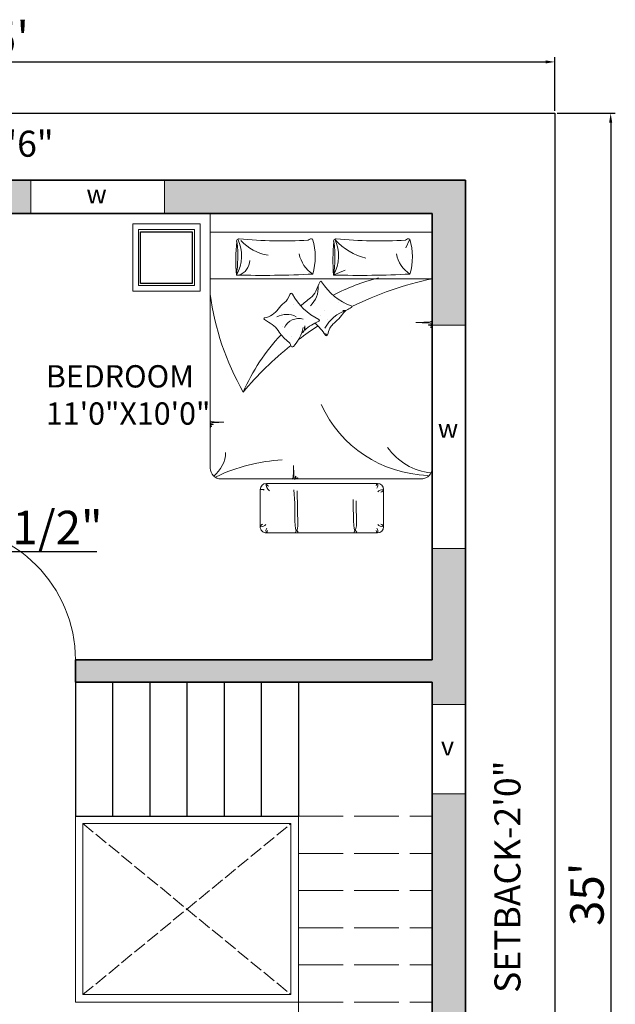
# Model space of a CAD drawing. Units: inches. Extents: x 3488 to 4319, y 780 to 1756.
# Tile 5 of 8: x 3679 to 3839, y 1491 to 1756. Entities that reach past the tile are written whole.
import ezdxf

# ---------------------------------------------------------------- set-up
doc = ezdxf.new("R2010")
doc.units = ezdxf.units.IN
doc.linetypes.add('ACAD_ISO02W100', pattern=[15, 12, -3])
for name, color, linetype, lineweight in [('A-ANNO-IDEN', 7, 'Continuous', 13), ('A-ANNO-TEXT', 7, 'Continuous', 18), ('A-AREA-IDEN', 7, 'Continuous', 18), ('A-DOOR', 4, 'Continuous', 18), ('A-FLOR-OPEN', 3, 'Continuous', 20), ('A-FLOR-OPEN-HIDN', 3, 'ACAD_ISO02W100', 13), ('A-FLOR-STRS', 7, 'Continuous', 25), ('A-FLOR-STRS-OVHD', 8, 'ACAD_ISO02W100', 18), ('A-WALL', 7, 'Continuous', 35), ('A-WALL-PATT', 252, 'Continuous', 13), ('C-PROP', 7, 'Continuous', 25), ('DIM', 9, 'Continuous', 18), ('FUR', 42, 'Continuous', 18), ('window', 130, 'Continuous', 18)]:
    doc.layers.add(name, color=color, linetype=linetype, lineweight=lineweight)
doc.layers.add('HA-FUR', color=8, linetype='Continuous')
doc.layers.add('wood', color=26, linetype='Continuous')
doc.styles.get("Standard").update_dxf_attribs({"font": 'arial.ttf'})
doc.dimstyles.new('ISO-25', dxfattribs={"dimtxt": 9, "dimasz": 2.5, "dimexe": 1.25, "dimexo": 0.625, "dimtad": 1, "dimdec": 1, "dimlunit": 3, "dimtxsty": 'Standard', "dimcen": 2.5, "dimclrd": 1, "dimclre": 1, "dimclrt": 1, "dimadec": 0, "dimazin": 0, "dimtfac": 1, "dimtdec": 1, "dimtmove": 0, "dimatfit": 3, "dimfxl": 1, "dimarcsym": 0})

# ---------------------------------------------------------------- blocks, each defined once
blk = doc.blocks.new('*U3')
for p, q in [((0, 0), (0, -6)), ((36, 0), (36, -6))]:
    blk.add_line(p, q)
blk.add_lwpolyline([(0, 0), (0, 36), (1.75, 36), (1.75, 0)], close=True)
blk.add_arc((0, 0), 36, 0, 90)
blk = doc.blocks.new('*D5')
at = {"layer": 'Defpoints', "color": 0, "transparency": 16777216}
for p in [(3822.99, 1744.35), (3522.99, 1730.55), (3822.99, 1730.55)]:
    blk.add_point(p, dxfattribs=at)
at = {"layer": 'DIM', "color": 0, "lineweight": -2, "transparency": 16777216}
for p, q in [((3522.99, 1731.18), (3522.99, 1745.6)), ((3822.99, 1731.18), (3822.99, 1745.6)), ((3525.49, 1744.35), (3820.49, 1744.35))]:
    blk.add_line(p, q, dxfattribs=at)
at = {"layer": 'DIM', "color": 0, "transparency": 16777216}
for points in [[(3525.49, 1744.77), (3525.49, 1743.94), (3522.99, 1744.35)], [(3820.49, 1744.77), (3820.49, 1743.94), (3822.99, 1744.35)]]:
    blk.add_solid(points, dxfattribs=at)
at = {"layer": 'DIM', "color": 0, "transparency": 16777216, "insert": (3672.99, 1749.57), "char_height": 9, "attachment_point": 5}
blk.add_mtext("25'", dxfattribs=at)
blk = doc.blocks.new('*D6')
at = {"layer": 'Defpoints', "color": 0, "transparency": 16777216}
for p in [(3822.99, 1730.55), (3822.99, 1310.55), (3838.01, 1310.55)]:
    blk.add_point(p, dxfattribs=at)
at = {"layer": 'DIM', "color": 0, "lineweight": -2, "transparency": 16777216}
for p, q in [((3823.61, 1730.55), (3839.26, 1730.55)), ((3838.01, 1728.05), (3838.01, 1313.05)), ((3823.61, 1310.55), (3839.26, 1310.55))]:
    blk.add_line(p, q, dxfattribs=at)
at = {"layer": 'DIM', "color": 0, "transparency": 16777216}
for points in [[(3837.59, 1728.05), (3838.43, 1728.05), (3838.01, 1730.55)], [(3837.59, 1313.05), (3838.43, 1313.05), (3838.01, 1310.55)]]:
    blk.add_solid(points, dxfattribs=at)
at = {"layer": 'DIM', "color": 0, "transparency": 16777216, "insert": (3832.79, 1520.55), "char_height": 9, "attachment_point": 5, "rotation": 90}
blk.add_mtext("35'", dxfattribs=at)
blk = doc.blocks.new('*X27')
at = {"color": 0}
for p, q in [((3147.8, 8143.4), (3147.8, 8143.4)), ((3155.9, 8182.9), (3155.9, 8182.9)), ((3209.5, 8023.9), (3209.5, 8023.9)), ((3251.6, 7997), (3251.6, 7997)), ((3283, 8049.6), (3283, 8049.6)), ((3154.1, 7950.7), (3154.1, 7950.7))]:
    blk.add_line(p, q, dxfattribs=at)
blk = doc.blocks.new('*X26')
at = {"color": 0}
for p, q in [((3155.9, 8182.9), (3155.9, 8182.9)), ((3139.8, 7939.7), (3139.8, 7939.7))]:
    blk.add_line(p, q, dxfattribs=at)
blk = doc.blocks.new('*X25')
at = {"color": 0}
for p, q in [((3155.9, 8182.9), (3155.9, 8182.9)), ((3139.8, 7939.7), (3139.8, 7939.7))]:
    blk.add_line(p, q, dxfattribs=at)
blk = doc.blocks.new('*X24')
at = {"color": 0}
for p, q in [((3163, 7776.2), (3163, 7776.2)), ((3422.2, 7761.3), (3422.2, 7761.3)), ((3236.2, 7675.7), (3236.2, 7675.7)), ((3244.3, 7698.6), (3244.3, 7698.6)), ((3340.3, 7689.4), (3340.3, 7689.4))]:
    blk.add_line(p, q, dxfattribs=at)
blk = doc.blocks.new('BED1')
for p, q in [((0, -1000), (0, 800)), ((150, 800), (0, 800)), ((150, 800), (150, -1000)), ((2058.7, 800), (150, 800)), ((528, 800), (528, -1000)), ((211.8, 614.9), (277.5, 585.4)), ((2537.2, 404.9), (2237.2, 404.9)), ((2187.2, 354.9), (2187.2, -545.1)), ((2587.2, -545.1), (2587.2, 354.9)), ((2566.3, 178.5), (2565.2, 177.4)), ((2582, 188.1), (2565.4, 174.8)), ((2565.4, 174.8), (2585.7, 165.4)), ((2566.3, -296.8), (2565.2, -297.9)), ((2582, -287.1), (2565.4, -300.5)), ((2565.4, -300.5), (2585.7, -309.9)), ((2237.2, -595.1), (2537.2, -595.1)), ((150, -1000), (0, -1000)), ((150, -1000), (2063.5, -1000))]:
    blk.add_line(p, q)
for points in [[(934, 797.9), (930.9, 797.7), (928.3, 797.4), (926.3, 796.9), (924.9, 796.3), (923.8, 795.6), (923.1, 794.8), (922.7, 793.8), (922.5, 792.7), (922.4, 791.5), (922.5, 790.3), (922.6, 789.2), (922.6, 788.3), (922.6, 787.6), (922.4, 787.3), (922, 787.4), (921.4, 787.9), (920.6, 788.9), (919.5, 790.2), (918.4, 791.6), (917.1, 793.1), (915.9, 794.6), (914.6, 796), (913.3, 797.1), (912.2, 797.9), (911.1, 798.3), (910.1, 798.4), (909.2, 798), (908.3, 797.1), (907.5, 795.8), (906.8, 793.9), (906, 791.4), (905.4, 788.5), (904.8, 785.2), (904.2, 781.7), (903.7, 778.4), (903.2, 775.4), (902.8, 772.9), (902.5, 771.3), (902.3, 770.6), (902.1, 771.2), (902, 772.8), (901.8, 775.2), (901.7, 778.1), (901.5, 781.5), (901.2, 785), (900.8, 788.4), (900.2, 791.5), (899.5, 794.1), (898.6, 796.2), (897.6, 797.9), (896.5, 799.2), (895.3, 800), (894.1, 800.5), (893, 800.7), (891.9, 800.5), (890.9, 800.1), (890, 799), (889.1, 797.1), (888.3, 794), (887.6, 789.3), (886.9, 782.9), (886.2, 774.2), (885.5, 763.1), (884.8, 749.5), (884.2, 734.2), (883.6, 718.3), (883, 702.8), (882.5, 688.8), (882, 677.5), (881.7, 669.8), (881.5, 666.9), (881.3, 669.4), (881.3, 676.7), (881.3, 687.8), (881.2, 701.5), (881.1, 716.8), (880.8, 732.6), (880.2, 748), (879.4, 761.8), (878.3, 773.2), (876.9, 782.2), (875.1, 789.2), (872.9, 794.4), (870.3, 798), (869, 799)], [(2150, -913.5), (2150, 723.2)], [(2327.6, 182.3), (2530, 185.9), (2550.8, 181.9), (2561.7, 179), (2566, 176.7), (2566.9, 174.4), (2566.3, 171.9), (2562, 169.2), (2550.3, 166.5), (2527.7, 163.9), (2490.6, 161.8), (2345.5, 160.2), (2317.8, 158.5)], [(494.7, 3.1), (458.9, 95.3)], [(2149.7, -259.9), (2150, -268.4), (2150.1, -274.1), (2150.1, -278.1), (2150, -281.4), (2149.8, -284), (2149.5, -286.1), (2149.1, -287.8), (2148.7, -289), (2148.1, -289.9), (2147.4, -290.5), (2146.6, -290.8), (2145.6, -291), (2144.6, -291), (2143.6, -291), (2142.7, -290.9), (2141.9, -290.9), (2141.4, -290.9), (2141.1, -291), (2141.2, -291.4), (2141.7, -291.9), (2142.5, -292.6), (2143.5, -293.4), (2144.7, -294.4), (2146, -295.4), (2147.2, -296.5), (2148.4, -297.6), (2149.3, -298.6), (2150, -299.6), (2150.3, -300.5), (2150.4, -301.3), (2150, -302.1), (2149.3, -302.8), (2148.2, -303.5), (2146.6, -304.1), (2144.6, -304.7), (2142.1, -305.2), (2139.3, -305.7), (2136.5, -306.2), (2133.7, -306.6), (2131.2, -307), (2129.2, -307.3), (2127.8, -307.6), (2127.3, -307.8), (2127.7, -308), (2129, -308.1), (2131, -308.2), (2133.5, -308.3), (2136.3, -308.5), (2139.2, -308.7), (2142, -309), (2144.6, -309.5), (2146.8, -310.1), (2148.6, -310.9), (2150, -311.7), (2151, -312.7), (2151.7, -313.6), (2152.1, -314.6), (2152.3, -315.6), (2152.2, -316.5), (2151.8, -317.3), (2150.9, -318.1), (2149.3, -318.8), (2146.7, -319.4), (2142.8, -320), (2137.4, -320.6), (2130.2, -321.2), (2121, -321.8), (2109.7, -322.3), (2096.9, -322.9), (2083.6, -323.4), (2070.7, -323.9), (2059.1, -324.3), (2049.6, -324.7), (2043.2, -325), (2040.8, -325.2), (2042.9, -325.3), (2049, -325.3), (2058.2, -325.3), (2069.6, -325.4), (2082.3, -325.5), (2095.6, -325.8), (2108.4, -326.2), (2119.9, -326.8), (2129.4, -327.8), (2136.9, -329), (2142.7, -330.5), (2147, -332.3), (2150, -334.4), (2150.9, -335.6)], [(2246.5, -294.4), (2530, -289.4), (2550.8, -293.4), (2561.7, -296.3), (2566, -298.6), (2566.9, -300.8), (2566.3, -303.4), (2562, -306.1), (2550.3, -308.8), (2527.7, -311.3), (2490.6, -313.5), (2345.5, -315), (2238.6, -321.8)], [(1733.7, -998.3), (1731.1, -998.1), (1729, -997.8), (1727.4, -997.4), (1726.1, -997), (1725.2, -996.4), (1724.7, -995.7), (1724.3, -994.8), (1724.1, -993.9), (1724.1, -992.9), (1724.1, -991.9), (1724.2, -991), (1724.2, -990.2), (1724.2, -989.7), (1724.1, -989.4), (1723.8, -989.5), (1723.2, -990), (1722.5, -990.8), (1721.7, -991.8), (1720.7, -993), (1719.7, -994.3), (1718.6, -995.5), (1717.5, -996.6), (1716.5, -997.6), (1715.5, -998.3), (1714.6, -998.6), (1713.8, -998.6), (1713, -998.3), (1712.3, -997.6), (1711.7, -996.5), (1711, -994.9), (1710.4, -992.9), (1709.9, -990.4), (1709.4, -987.6), (1708.9, -984.8), (1708.5, -982), (1708.1, -979.5), (1707.8, -977.4), (1707.5, -976.1), (1707.3, -975.5), (1707.1, -976), (1707, -977.3), (1706.9, -979.3), (1706.8, -981.8), (1706.7, -984.6), (1706.4, -987.5), (1706.1, -990.3), (1705.6, -992.9), (1705, -995.1), (1704.2, -996.9), (1703.4, -998.3), (1702.4, -999.3), (1701.5, -1000), (1700.5, -1000.4), (1699.6, -1000.6), (1698.7, -1000.4), (1697.8, -1000.1), (1697, -999.2), (1696.3, -997.6), (1695.7, -995), (1695.1, -991.1), (1694.5, -985.7), (1693.9, -978.5), (1693.3, -969.3), (1692.8, -957.9), (1692.2, -945.2), (1691.7, -931.9), (1691.2, -919), (1690.8, -907.4), (1690.4, -897.9), (1690.1, -891.5), (1689.9, -889.1), (1689.8, -891.2), (1689.8, -897.3), (1689.8, -906.5), (1689.7, -917.9), (1689.6, -930.6), (1689.4, -943.8), (1688.9, -956.6), (1688.3, -968.1), (1687.3, -977.6), (1686.1, -985.2), (1684.6, -991), (1682.8, -995.3), (1680.7, -998.3), (1679.6, -999.2)]]:
    blk.add_lwpolyline(points)
for points in [[(489.2, 619.6, 0.144019), (207.6, 617.9, 0.248643)], [(205.5, 619.6, 0.267769), (215.1, 582.4, -0.037739), (204.3, 21.8, 0.684696), (236.7, 5.5, -0.060702), (497.2, 0.1, -0.046649), (225.9, 3.1, -1.318436)], [(497.2, 0.1, 0.021276), (489.2, 619.6, -0.206383), (326.6, 509.4, 0.237198)], [(211.8, 12.8, 0.143972), (361.6, 262.9, 1.292232)], [(886.4, -150, -0.069098), (985, -66.5, 0.658965), (982.1, -48.7, -0.049789), (927.4, -29, -0.103757), (896.6, -5.4, 0.055725), (800.9, 83.3, -0.11866), (782.7, 104.9, 0.016811), (761.6, 143.9, 0.70791), (748.3, 144, -0.16964), (551.9, -96.6, 0.664036), (554, -110.7, 0.023706), (627, -144.7, -0.134834), (683.2, -188, 0.012748), (746.3, -267.4)], [(489.2, -168.2, 0.144019), (207.6, -169.9, 0.248643)], [(969.1, -259.1, 0.263265), (936.3, -236.9, -0.026108), (909.2, -233.2, 0.027613), (945.1, -234.2, -0.089259), (872.7, -120, 0.662242), (857.6, -119.3, -0.162037), (651.8, -332.7, 0.676499), (654, -354.5, -0.160513), (722.9, -401.5, 0.07473), (773.5, -450.3, -0.187721), (845.5, -559.9, 0.70791), (858.8, -561.4, -0.010003), (898.6, -497.3, -0.113819), (947.3, -450.2, 0.099539), (1032.5, -372.4, -0.173425), (1070.9, -346.4, 0.589988), (1076.2, -326.1, 0.137312), (923.9, -245.9, 0.137312)], [(205.5, -168.2, 0.267769), (215.1, -205.4, -0.037739), (204.3, -766, 0.684696), (236.7, -782.3, -0.060702), (497.2, -787.7, -0.046649), (225.9, -784.7, -1.318436)], [(497.2, -787.7, 0.021276), (489.2, -168.2, -0.206383), (326.6, -278.4, 0.237198)], [(1446, -733.4, -0.095039), (652.8, -1001.7)]]:
    blk.add_lwpolyline(points, format="xyb")
for centre, radius, start, end in [((3208.8, 1363.3), 2739.4, 191.86791, 206.32469), ((2062.7, 713.7), 86.5, 0, 93.53765), ((1138.6, 793.9), 983.2, 294.60777, 358.30329), ((1608.1, 842.5), 496.3, 305.19014, 354.02057), ((2237.2, 354.9), 50, 90, 180), ((2321.1, 409.7), 84.5, 185.61958, 217.13957), ((2227.5, 373.5), 32.8, 17.83305, 72.80048), ((2546.9, 373.5), 32.8, 107.19952, 162.16695), ((2453.3, 409.7), 84.5, 322.86043, 354.38042), ((2537.2, 354.9), 50, 0, 90), ((2098.7, 754.7), 1625, 193.90497, 207.81692), ((2201.9, 323.3), 34.8, 50.8413, 114.9586), ((2212.2, 381.5), 36.5, 226.80948, 258.3841), ((2572.5, 323.3), 34.8, 65.0414, 129.1587), ((2562.2, 381.5), 36.5, 281.6159, 313.19052), ((751.8, 88.7), 34.9, 336.83517, 27.72181), ((684.2, 86), 100.3, 353.675, 10.88198), ((1074.1, 198.8), 306.1, 197.86019, 241.51221), ((341.4, -277.7), 318.5, 60.71255, 115.00895), ((983.7, -79.5), 20.8, 73.79673, 130.45661), ((978.5, -68.6), 14.3, 39.7097, 85.9506), ((602.5, -324), 198.6, 43.20348, 95.05559), ((3208.8, 1363.3), 2739.4, 212.93136, 216.95099), ((980, -379), 163.4, 152.61037, 209.36102), ((981.1, -281.8), 131.1, 164.0372, 243.45361), ((3208.8, 1363.3), 2739.4, 218.63292, 229.94485), ((2098.7, 754.7), 1625, 226.58872, 246.3156), ((3402.5, -342.9), 1408.5, 182.99169, 205.68187), ((-34.4, -471.2), 376.5, 312.01178, 350.96348), ((2178, -513.5), 33, 286.18268, 338.13858), ((2237.2, -545.1), 50, 180, 270), ((2188.1, -476.2), 73, 269.45125, 322.80265), ((2453.3, -600), 84.5, 5.61958, 37.13957), ((2537.2, -545.1), 50, 270, 0), ((2572.5, -513.6), 34.8, 230.8413, 294.9586), ((2562.2, -571.8), 36.5, 46.80948, 78.3841), ((2271.1, -580.9), 35.8, 148.90546, 197.55407), ((2546.9, -563.8), 32.8, 197.83305, 252.80048), ((375.7, -807.4), 128.2, 17.40732, 88.51286), ((341.4, -1065.5), 318.5, 60.71255, 115.00895), ((1929.1, -1126), 250.5, 37.85533, 88.44053), ((2063.5, -913.5), 86.5, 270, 0)]:
    blk.add_arc(centre, radius, start, end)
for name in ['*X26', '*X25', '*X27', '*X24']:
    blk.add_blockref(name, (-2425.3, -8101.4))
blk = doc.blocks.new('A$C647F3D92')
at = {"layer": 'FUR'}
for points in [[(0.6, 0.6), (0, 0.6), (0, 0), (0.6, 0)], [(0.55, 0.55), (0.05, 0.55), (0.05, 0.05), (0.55, 0.05)]]:
    blk.add_lwpolyline(points, close=True, dxfattribs=at)
at = {"layer": 'HA-FUR'}
blk.add_lwpolyline([(0.53, 0.53), (0.07, 0.53), (0.07, 0.07), (0.53, 0.07)], close=True, dxfattribs=at)
blk = doc.blocks.new('A$C38A85F6B')
at = {"layer": 'wood', "xscale": -1, "rotation": 359.9999999999109}
blk.add_blockref('A$C647F3D92', (0.6, 0), dxfattribs=at)
blk = doc.blocks.new('STAIR-GROUND-LOWER-FLIGHT')
for p, q in [((0, 36), (0, 0)), ((10, 36), (10, 0)), ((20, 36), (20, 0)), ((30, 36), (30, 0)), ((40, 36), (40, 0)), ((50, 36), (50, 0)), ((60, 36), (60, 0)), ((0, 0), (60, 0))]:
    blk.add_line(p, q)
blk = doc.blocks.new('STAIR-GROUND-OVERHEAD-FLIGHT')
for p, q in [((0, 86), (0, 0)), ((0, 86), (36, 86)), ((0, 76), (36, 76)), ((0, 66), (36, 66)), ((0, 56), (36, 56)), ((0, 46), (36, 46)), ((0, 36), (36, 36)), ((0, 0), (36, 0))]:
    blk.add_line(p, q)
blk = doc.blocks.new('OPENING-STAIRWELL-FRAME')
for points in [[(60, 50), (0, 50), (0, 0), (60, 0)], [(58, 48), (2, 48), (2, 2), (58, 2)]]:
    blk.add_lwpolyline(points, close=True)
blk = doc.blocks.new('*D91')
at = {"layer": 'Defpoints', "color": 0, "transparency": 16777216}
for p in [(3630.4, 1616.73), (3651.99, 1616.73), (3651.99, 1612.71)]:
    blk.add_point(p, dxfattribs=at)
at = {"layer": 'DIM', "color": 1, "lineweight": -2, "transparency": 16777216}
for p, q in [((3630.4, 1616.1), (3630.4, 1611.46)), ((3651.99, 1616.1), (3651.99, 1611.46)), ((3632.9, 1612.71), (3649.49, 1612.71)), ((3651.99, 1612.71), (3699.79, 1612.71))]:
    blk.add_line(p, q, dxfattribs=at)
at = {"layer": 'DIM', "color": 1, "transparency": 16777216}
for points in [[(3632.9, 1613.13), (3632.9, 1612.29), (3630.4, 1612.71)], [(3649.49, 1613.13), (3649.49, 1612.29), (3651.99, 1612.71)]]:
    blk.add_solid(points, dxfattribs=at)
at = {"layer": 'DIM', "color": 1, "transparency": 16777216, "insert": (3677.14, 1617.99), "char_height": 9, "attachment_point": 5}
blk.add_mtext('1\'-9 1/2"', dxfattribs=at)

msp = doc.modelspace()

# ---------------------------------------------------------------- hatches: boundary and pattern name
at = {"layer": 'A-WALL-PATT', "transparency": 33554687}
h = msp.add_hatch(color=256, dxfattribs=at)
h.dxf.hatch_style = 1
h.paths.add_polyline_path([(3657.99, 1505.55), (3657.99, 1535.55), (3651.99, 1535.55), (3651.99, 1505.55), (3609.99, 1505.55), (3609.99, 1544.55), (3603.99, 1544.55), (3603.99, 1505.55), (3555.99, 1505.55), (3555.99, 1514.55), (3546.99, 1514.55), (3546.99, 1496.55), (3648.99, 1496.55), (3648.99, 1352.55), (3663.99, 1352.55), (3663.99, 1361.55), (3657.99, 1361.55)])
h.paths.add_polyline_path([(3722.99, 1361.55), (3719, 1361.55), (3703.99, 1361.55), (3703.99, 1352.55), (3722.99, 1352.55)])
h.paths.add_polyline_path([(3798.99, 1397.55), (3789.99, 1397.55), (3789.99, 1361.95), (3789.99, 1361.55), (3770.99, 1361.55), (3770.99, 1352.55), (3798.99, 1352.55)])
h.paths.add_polyline_path([(3798.99, 1547.58), (3789.99, 1547.58), (3789.99, 1463.55), (3798.99, 1463.55)])
h.paths.add_polyline_path([(3798.99, 1613.55), (3789.99, 1613.55), (3789.99, 1583.55), (3693.99, 1583.55), (3693.99, 1577.55), (3789.99, 1577.55), (3789.99, 1571.58), (3798.99, 1571.58)])
h.paths.add_polyline_path([(3798.99, 1712.55), (3717.99, 1712.55), (3717.99, 1703.55), (3789.99, 1703.55), (3789.99, 1673.55), (3798.99, 1673.55)])
h.paths.add_polyline_path([(3681.99, 1712.55), (3627.99, 1712.55), (3627.99, 1703.55), (3651.99, 1703.55), (3651.99, 1577.55), (3657.99, 1577.55), (3657.99, 1703.55), (3681.99, 1703.55)])
h.paths.add_polyline_path([(3591.99, 1712.55), (3546.99, 1712.55), (3546.99, 1667.55), (3555.99, 1667.55), (3555.99, 1703.55), (3591.99, 1703.55)])
edge = h.paths.add_edge_path()
edge.add_line((3555.99, 1619.55), (3546.99, 1619.55))
edge.add_line((3546.99, 1619.55), (3546.99, 1538.55))
edge.add_line((3546.99, 1538.55), (3555.99, 1538.55))
edge.add_line((3555.99, 1538.55), (3555.99, 1565.03))
edge.add_ellipse((3556.27, 1565.11), major_axis=(0.21, 0.21), ratio=0.999043, start_angle=135, end_angle=151.1563, ccw=False)
edge.add_line((3555.98, 1565.08), (3555.99, 1577.26))
edge.add_line((3555.99, 1577.26), (3555.99, 1577.55))
edge.add_line((3555.99, 1577.55), (3603.99, 1577.55))
edge.add_line((3603.99, 1577.55), (3603.99, 1574.55))
edge.add_line((3603.99, 1574.55), (3609.99, 1574.55))
edge.add_line((3609.99, 1574.55), (3609.99, 1583.55))
edge.add_line((3609.99, 1583.55), (3555.99, 1583.55))
edge.add_line((3555.99, 1583.55), (3555.99, 1619.55))

# ---------------------------------------------------------------- linework, layer by layer
at = {"layer": 'A-FLOR-OPEN-HIDN', "ltscale": 0.3}
for p, q in [((3695.99, 1539.55), (3751.99, 1493.55)), ((3695.99, 1493.55), (3751.99, 1539.55))]:
    msp.add_line(p, q, dxfattribs=at)
at = {"layer": 'A-WALL'}
for p, q in [((3546.99, 1712.55), (3798.99, 1712.55)), ((3798.99, 1712.55), (3798.99, 1352.55)), ((3657.99, 1703.55), (3789.99, 1703.55)), ((3789.99, 1703.55), (3789.99, 1583.55)), ((3693.99, 1583.55), (3693.99, 1577.55)), ((3693.99, 1583.55), (3789.99, 1583.55)), ((3693.99, 1577.55), (3789.99, 1577.55)), ((3789.99, 1577.55), (3789.99, 1361.55))]:
    msp.add_line(p, q, dxfattribs=at)
at = {"layer": 'C-PROP'}
for p, q in [((3522.99, 1730.55), (3822.99, 1730.55)), ((3822.99, 1730.55), (3822.99, 1310.55))]:
    msp.add_line(p, q, dxfattribs=at)
at = {"layer": 'window'}
for p, q in [((3681.99, 1703.55), (3681.99, 1712.55)), ((3717.99, 1703.55), (3717.99, 1712.55)), ((3789.99, 1673.55), (3798.99, 1673.55)), ((3789.99, 1613.55), (3798.99, 1613.55)), ((3789.99, 1571.58), (3798.99, 1571.58)), ((3789.99, 1547.58), (3798.99, 1547.58))]:
    msp.add_line(p, q, dxfattribs=at)

# ---------------------------------------------------------------- block references
at = {"layer": 'A-DOOR'}
msp.add_blockref('*U3', (3657.99, 1583.55), dxfattribs=at)
at = {"layer": 'A-FLOR-OPEN'}
msp.add_blockref('OPENING-STAIRWELL-FRAME', (3693.99, 1491.55), dxfattribs=at)
at = {"layer": 'A-FLOR-STRS'}
msp.add_blockref('STAIR-GROUND-LOWER-FLIGHT', (3693.99, 1541.55), dxfattribs=at)
at = {"layer": 'A-FLOR-STRS-OVHD'}
msp.add_blockref('STAIR-GROUND-OVERHEAD-FLIGHT', (3753.99, 1455.55), dxfattribs=at)
at = {"layer": 'FUR', "xscale": 0.0331718847221821, "yscale": 0.0331718847221821, "zscale": 0.0331718847221821, "rotation": 270}
msp.add_blockref('BED1', (3763.45, 1703.55), dxfattribs=at)
at = {"layer": 'FUR', "xscale": 30.18374333319767, "yscale": 30.18374333319767, "zscale": 30.18374333319767}
msp.add_blockref('A$C38A85F6B', (3709.41, 1682.69), dxfattribs=at)

# ---------------------------------------------------------------- texts
at = {"layer": 'A-ANNO-IDEN'}
for s, p in [('w', (3696.94, 1706.3)), ('w', (3791.51, 1643.28)), ('v', (3792.33, 1557.87))]:
    msp.add_text(s, height=5, dxfattribs=at).set_placement(p)
at = {"layer": 'A-ANNO-TEXT', "insert": (3625.66, 1725.86), "char_height": 7, "attachment_point": 1}
msp.add_mtext_dynamic_manual_height_columns('\\pxt7;{SETBACK-1\'6"}', width=83.4163, gutter_width=25, heights=[0], dxfattribs=at)
at = {"layer": 'A-ANNO-TEXT', "insert": (3806.74, 1494.03), "char_height": 7, "attachment_point": 1, "rotation": 90}
msp.add_mtext_dynamic_manual_height_columns('\\pxt7;{SETBACK-2\'0"}', width=83.4163, gutter_width=25, heights=[0], dxfattribs=at)
at = {"layer": 'A-AREA-IDEN', "insert": (3686.05, 1662.81), "char_height": 6, "attachment_point": 1}
msp.add_mtext_dynamic_manual_height_columns('BEDROOM\\P11\'0"X10\'0"', width=83.4163, gutter_width=25, heights=[0], dxfattribs=at)

# ---------------------------------------------------------------- dimensions: what is measured, and where the dimension line sits
at = {"layer": 'DIM'}
for base, p1, p2, override, picture, middle in [((3822.99, 1744.35), (3522.99, 1730.55), (3822.99, 1730.55), {"dimclrd": 0, "dimclre": 0, "dimclrt": 0}, '*D5', (3672.99, 1749.57)), ((3651.99, 1612.71), (3630.4, 1616.73), (3651.99, 1616.73), {"dimdec": 1, "dimlfac": 1, "dimrnd": 0, "dimzin": 1, "dimdsep": 46, "dimlunit": 4, "dimfrac": 2}, '*D91', (3677.14, 1617.99))]:
    dim = msp.add_linear_dim(base=base, p1=p1, p2=p2, dimstyle='ISO-25', override=override, dxfattribs=at)
    dim.commit()
    dim.dimension.update_dxf_attribs({"geometry": picture, "text_midpoint": middle})
dim = msp.add_linear_dim(base=(3838.01, 1310.55), p1=(3822.99, 1730.55), p2=(3822.99, 1310.55), angle=90, dimstyle='ISO-25', override={"dimclrd": 0, "dimclre": 0, "dimclrt": 0}, dxfattribs=at)
dim.commit()
dim.dimension.update_dxf_attribs({"geometry": '*D6', "text_midpoint": (3832.79, 1520.55)})

doc.saveas('drawing.dxf')
